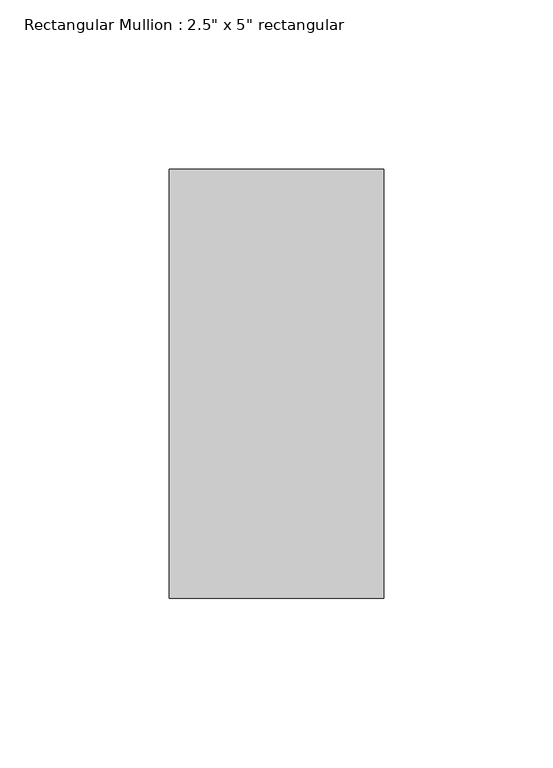
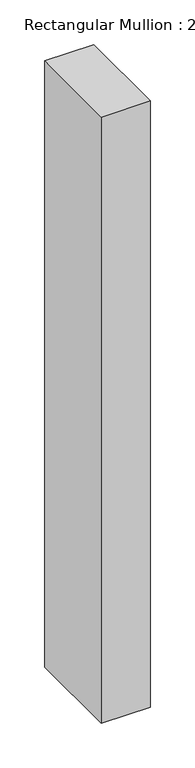
"""IFC4 building model written with IfcOpenShell, lengths in millimetres: member geometry."""

from ifc_helpers import new_model, si_unit, frame, origin, place, context, project, spatial, polyline, outline, extrude, source, transform, mapped, element, save


def member_171fbd6b(model_context):
    return source(origin(), model_context, "Body", "SweptSolid", [
        extrude(outline(polyline([(0.0, 63.5), (0.0, -63.5), (-63.5, -63.5), (-63.5, 63.5), (0.0, 63.5)])), frame((0.0, 0.0, -830.6744987), z_axis=(0.0, 0.0, 1.0), x_axis=(1.0, 0.0, 0.0)), (0.0, 0.0, 1.0), 830.6744987),
    ])


if __name__ == "__main__":
    model = new_model("IFC4")
    model_context = context("Model", 3, world=origin())
    ifc_project = project(units=[si_unit("LENGTHUNIT", "METRE", prefix="MILLI")], contexts=[model_context])
    site = spatial("IfcSite", under=ifc_project)
    building = spatial("IfcBuilding", under=site)
    placement = place(None, origin())
    member_shape = member_171fbd6b(model_context)
    element("IfcMember", 1, ObjectType="Rectangular Mullion : 2.5\" x 5\" rectangular", at=placement, inside=building, context=model_context, shape_type="MappedRepresentation", body=[
        mapped(member_shape, transform((0.0, 0.0, 0.0), x_axis=(1.0, 0.0, 0.0), y_axis=(0.0, 1.0, 0.0), z_axis=(0.0, 0.0, 1.0))),
    ])
    save(model, "model.ifc")

# Revit data of these elements
# Type "Rectangular Mullion : 2.5\" x 5\" rectangular"
#   built-in parameter 1007304 = 0.416667 (stored number, unit not read)
#   built-in parameter 1007301 = 0.104167 (stored number, unit not read)
#   built-in parameter 1007300 = 0.104167 (stored number, unit not read)
# Element 1 (IfcMember, "Rectangular Mullion : 2.5\" x 5\" rectangular")
#   Materials on its faces: "Aluminum"
# Materials
#   "Aluminum": class "Metal", colour RGB 247 247 247, transparency 0, Description = "Aluminum 6061", Cost = 0
